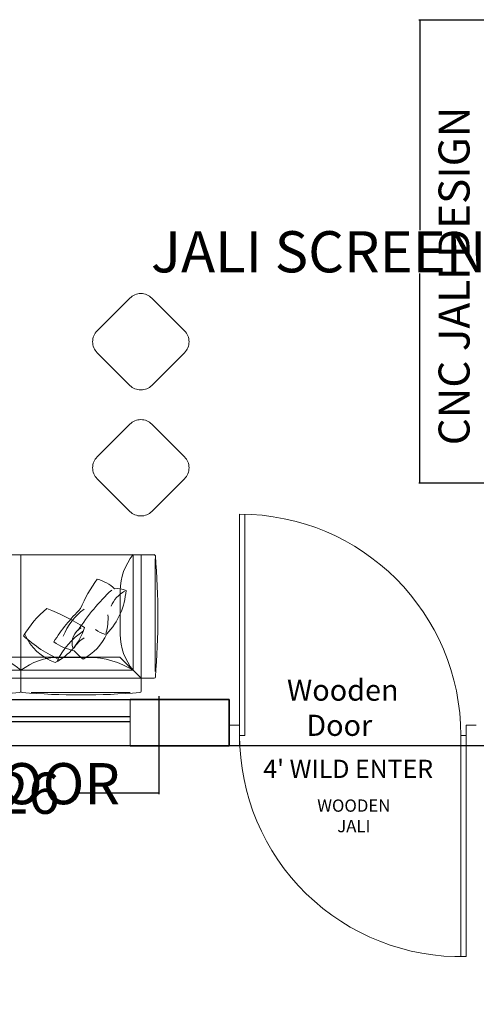
# Model space of a CAD drawing. Units: inches. Extents: x -48 to 50072, y 0 to 21068.
# Tile 50 of 75: x 123 to 212, y 628 to 819. Entities that reach past the tile are written whole.
import ezdxf

# ---------------------------------------------------------------- set-up
doc = ezdxf.new("R2010")
doc.units = ezdxf.units.IN
doc.header["$MEASUREMENT"] = 0
for name, color, linetype, lineweight in [('A-ANNO-DIMS', 2, 'Continuous', 18), ('A-ANNO-TEXT', 7, 'Continuous', 18), ('A-DOOR', 4, 'Continuous', 18), ('A-WALL', 7, 'Continuous', 35), ('FURNITURE', 44, 'Continuous', 18)]:
    doc.layers.add(name, color=color, linetype=linetype, lineweight=lineweight)
doc.layers.add('Layer3', color=176, linetype='Continuous')
doc.styles.get("Standard").update_dxf_attribs({"font": 'arial.ttf'})
doc.dimstyles.get("Standard").update_dxf_attribs({"dimtxt": 8, "dimasz": 0.18, "dimexe": 0.18, "dimexo": 0.0625, "dimgap": 0.09, "dimtad": 0, "dimtih": 1, "dimtoh": 1, "dimdec": 1, "dimzin": 0, "dimdsep": 46, "dimlunit": 4, "dimtxsty": 'Standard', "dimblk": 'ARCHTICK', "dimcen": 0.09, "dimadec": 0, "dimazin": 0, "dimtfac": 1, "dimtdec": 1, "dimtofl": 0, "dimtmove": 0, "dimatfit": 3, "dimldrblk": 'ARCHTICK', "dimfxl": 1, "dimtolj": 1, "dimtzin": 0, "dimarcsym": 0})

# ---------------------------------------------------------------- blocks, each defined once
blk = doc.blocks.new('fdsghhhhhhygr')
for p, q in [((41.77, 686.77), (41.77, 677.77)), ((144.77, 677.77), (144.77, 686.77))]:
    blk.add_line(p, q)
at = {"layer": 'Defpoints'}
for p, q in [((91.27, 683.47), (144.77, 683.47)), ((91.27, 683.47), (91.27, 682.47)), ((41.77, 682.07), (95.27, 682.07)), ((91.27, 682.47), (144.77, 682.47)), ((95.27, 682.07), (95.27, 681.07)), ((41.77, 681.07), (95.27, 681.07))]:
    blk.add_line(p, q, dxfattribs=at)
at = {"layer": 'Layer3'}
for p, q in [((41.77, 686.77), (144.77, 686.77)), ((144.77, 677.77), (41.77, 677.77))]:
    blk.add_line(p, q, dxfattribs=at)
blk = doc.blocks.new('WRG')
at = {"layer": 'FURNITURE'}
for centre, radius, start, end in [((-5881.03, 869.32), 50.97, 111.3371, 122.4176), ((-5914.7, 898.39), 23.82, 30.3068, 50.5663), ((-5895.33, 916.33), 13.61, 197.0126, 242.9429), ((-5918.49, 896.36), 18.43, 25.9005, 55.6513), ((-5915.78, 934.22), 32.17, 294.0815, 312.2768), ((-5905.57, 915.66), 12.15, 289.4501, 336.7699)]:
    blk.add_arc(centre, radius, start, end, dxfattribs=at)
blk = doc.blocks.new('DFGS')
at = {"layer": 'FURNITURE'}
for centre, radius, start, end in [((-6087.14, 813.36), 9.64, 104.9394, 132.5633), ((-6112.38, 805.26), 28.66, 21.6133, 37.4184), ((-6094.33, 816.04), 4.48, 81.3108, 116.3418), ((-6080.05, 821.2), 16.31, 184.0297, 223.6176), ((-6099.45, 813.66), 7.12, 22.214, 60.8038), ((-6126.91, 783.89), 49.66, 32.8076, 46.9), ((-6094.76, 804.41), 13.97, 20.7975, 53.8819), ((-6116.99, 784.16), 44.49, 32.4999, 45.375), ((-6080.96, 813.35), 11.17, 174.5959, 197.1556), ((-6092.61, 815.13), 5.43, 281.6061, 309.1892), ((-6087.9, 807.73), 4.17, 346.5527, 60.4145), ((-6080.21, 815.37), 12.85, 204.9913, 241.6537), ((-6089.91, 803.33), 6.58, 30.5945, 59.6065), ((-6086.56, 817.99), 12.2, 280.9279, 305.5545), ((-6095.16, 815.51), 14.47, 307.7029, 318.9387)]:
    blk.add_arc(centre, radius, start, end, dxfattribs=at)
blk = doc.blocks.new('3+2 seater sofa')
at = {"layer": 'FURNITURE'}
for p, q in [((1464.23, 900.93), (1464.23, 875.06)), ((1465.03, 901.17), (1486.94, 901.17)), ((1488.22, 900.95), (1488.22, 898.4)), ((1488.22, 898.4), (1464.22, 898.4)), ((1488.22, 898.4), (1484.13, 894.31)), ((1490.75, 898.4), (1488.22, 898.4)), ((1488.22, 898.4), (1488.22, 875.06, 0)), ((1486.69, 896.88), (1464.22, 896.88)), ((1486.69, 896.88), (1486.69, 875.06)), ((1490.98, 877.03), (1490.98, 896.27)), ((1484.13, 894.31, 0), (1464.22, 894.31)), ((1471.21, 894.37), (1479.69, 894.37)), ((1484.13, 894.31), (1484.13, 875.06)), ((1484.18, 888.22), (1484.18, 882.36)), ((1490.74, 875.06), (1464.23, 875.06)), ((1484.13, 875.06), (1490.75, 875.06)), ((1486.69, 863.06), (1486.69, 875.06)), ((1488.23, 851.03, 0), (1488.23, 875.06)), ((1490.98, 872.68), (1490.98, 863.06)), ((1484.15, 868.83), (1484.15, 863.06)), ((1484.15, 857.29), (1484.15, 863.06)), ((1484.15, 863.06, 0), (1484.15, 851.06)), ((1486.69, 863.06), (1486.69, 851.06)), ((1490.98, 853.57), (1490.98, 863.06)), ((1490.74, 851.06), (1464.23, 851.06)), ((1484.13, 851.06), (1490.75, 851.06)), ((1486.69, 839.06), (1486.69, 851.06)), ((1488.23, 827.03, 0), (1488.23, 851.06)), ((1490.98, 848.68), (1490.98, 839.06)), ((1484.15, 844.83), (1484.15, 839.06)), ((1484.15, 833.29), (1484.15, 839.06)), ((1484.15, 839.06, 0), (1484.15, 827.06)), ((1486.69, 839.06), (1486.69, 827.06)), ((1490.98, 829.57), (1490.98, 839.06)), ((1366.35, 827.06), (1392.23, 827.06)), ((1368.88, 803.07), (1368.88, 827.07)), ((1370.4, 804.59), (1370.4, 827.07)), ((1392.23, 800.54), (1392.23, 827.06)), ((1392.23, 800.54), (1392.23, 827.06)), ((1416.23, 800.54), (1416.23, 827.06)), ((1440.23, 800.54), (1440.23, 827.06)), ((1464.23, 800.54), (1464.23, 827.06)), ((1490.74, 827.06), (1464.23, 827.06)), ((1484.13, 827.06), (1490.75, 827.06)), ((1366.11, 826.25), (1366.11, 804.34)), ((1372.92, 820.07), (1372.92, 811.59)), ((1368.88, 803.07), (1372.97, 807.16)), ((1372.97, 807.16), (1392.23, 807.16)), ((1379.07, 807.11), (1384.92, 807.11)), ((1392.23, 807.16), (1392.23, 800.53)), ((1392.23, 807.16), (1392.23, 800.53)), ((1398.46, 807.13), (1404.23, 807.13)), ((1410, 807.13), (1404.23, 807.13)), ((1404.23, 807.13, 0), (1416.23, 807.13)), ((1416.23, 807.16), (1416.23, 800.53)), ((1422.46, 807.13), (1428.23, 807.13)), ((1434, 807.13), (1428.23, 807.13)), ((1428.23, 807.13, 0), (1440.23, 807.13)), ((1440.23, 807.16), (1440.23, 800.53)), ((1446.46, 807.13), (1452.23, 807.13)), ((1458, 807.13), (1452.23, 807.13)), ((1452.23, 807.13, 0), (1464.23, 807.13)), ((1464.23, 807.16), (1464.23, 800.53)), ((1370.4, 804.59), (1392.23, 804.59)), ((1404.23, 804.59), (1392.23, 804.59)), ((1404.23, 804.59), (1416.23, 804.59)), ((1428.23, 804.59), (1416.23, 804.59)), ((1428.23, 804.59), (1440.23, 804.59)), ((1452.23, 804.59), (1440.23, 804.59)), ((1452.23, 804.59), (1464.23, 804.59)), ((1366.33, 803.07), (1368.88, 803.07)), ((1368.88, 800.53), (1368.88, 803.07)), ((1368.88, 803.07), (1392.23, 803.07, 0)), ((1416.26, 803.06, 0), (1392.23, 803.06)), ((1440.26, 803.06, 0), (1416.23, 803.06)), ((1464.26, 803.06, 0), (1440.23, 803.06)), ((1390.25, 800.3), (1371.02, 800.3)), ((1394.6, 800.3), (1404.23, 800.3)), ((1413.72, 800.3), (1404.23, 800.3)), ((1418.6, 800.3), (1428.23, 800.3)), ((1437.72, 800.3), (1428.23, 800.3)), ((1442.6, 800.3), (1452.23, 800.3)), ((1461.72, 800.3), (1452.23, 800.3))]:
    blk.add_line(p, q, dxfattribs=at)
at = {"layer": 'FURNITURE', "ltscale": 3}
for p, q in [((1464.23, 875.06), (1464.23, 851.06)), ((1484.15, 863.06), (1484.15, 875.06)), ((1484.15, 863.06), (1484.15, 851.06)), ((1464.23, 851.06), (1464.23, 827.06)), ((1484.15, 839.06), (1484.15, 851.06)), ((1484.15, 839.06), (1484.15, 827.06)), ((1392.23, 827.06), (1416.23, 827.06)), ((1416.23, 827.06), (1440.23, 827.06)), ((1440.23, 827.06), (1464.23, 827.06)), ((1404.23, 807.13), (1392.23, 807.13)), ((1404.23, 807.13), (1416.23, 807.13)), ((1428.23, 807.13), (1416.23, 807.13)), ((1428.23, 807.13), (1440.23, 807.13)), ((1452.23, 807.13), (1440.23, 807.13)), ((1452.23, 807.13), (1464.23, 807.13))]:
    blk.add_line(p, q, dxfattribs=at)
at = {"layer": 'FURNITURE'}
for centre, radius, start, end in [((1476.31, 758.13), 143.55, 85.3368, 94.7395), ((1464.47, 900.93), 0.255, 94.7915, 180), ((1487.96, 900.95), 0.255, 0, 85.2857), ((1490.75, 898.15), 0.255, 5.7807, 90), ((1354.3, 886.73), 137.18, 355.2142, 4.7858), ((1471.31, 905.62), 11.26, 230.9515, 269.5157), ((1479.6, 905.62), 11.26, 270.4843, 309.0485), ((1500.6, 888.15), 16.42, 147.8787, 179.7559), ((1496.3, 882.45), 12.13, 180.424, 217.563), ((1493.43, 868.68), 9.28, 136.5598, 179.0844), ((1490.74, 874.8), 0.255, 4.5067, 90), ((1490.75, 875.31), 0.255, 270, 354.2193), ((1348.3, 862.96), 143.19, 0.0378, 4.7508), ((1348.3, 863.15), 143.19, 355.2492, 359.9622), ((1493.43, 857.43), 9.28, 180.9156, 223.4402), ((1493.43, 844.68), 9.28, 136.5598, 179.0844), ((1490.74, 851.31), 0.255, 270, 355.4933), ((1348.3, 838.96), 143.19, 0.0378, 4.7508), ((1348.3, 839.15), 143.19, 355.2492, 359.9622), ((1493.43, 833.43), 9.28, 180.9156, 223.4402), ((1509.16, 814.97), 143.55, 175.2605, 184.6632), ((1366.35, 826.81), 0.255, 90, 175.2085), ((1361.66, 819.98), 11.26, 0.4843, 39.0485), ((1490.74, 827.31), 0.255, 270, 355.4933), ((1361.66, 811.68), 11.26, 320.9515, 359.5157), ((1379.14, 790.68), 16.42, 90.2441, 122.1213), ((1384.83, 794.98), 12.13, 52.437, 89.576), ((1398.61, 797.86), 9.28, 90.9156, 133.4402), ((1409.85, 797.86), 9.28, 46.5598, 89.0844), ((1422.61, 797.86), 9.28, 90.9156, 133.4402), ((1433.85, 797.86), 9.28, 46.5598, 89.0844), ((1446.61, 797.86), 9.28, 90.9156, 133.4402), ((1457.85, 797.86), 9.28, 46.5598, 89.0844), ((1366.33, 803.32), 0.255, 184.7143, 270), ((1369.13, 800.53), 0.255, 180, 264.2193), ((1380.55, 936.98), 137.18, 265.2142, 274.7858), ((1391.97, 800.54), 0.255, 274.5067, 0), ((1391.97, 800.53), 0.255, 275.7807, 0), ((1392.48, 800.54), 0.255, 180, 265.4933), ((1392.48, 800.53), 0.255, 180, 264.2193), ((1404.32, 942.98), 143.19, 265.2492, 269.9622), ((1404.13, 942.98), 143.19, 270.0378, 274.7508), ((1415.97, 800.54), 0.255, 274.5067, 0), ((1428.32, 942.98), 143.19, 265.2492, 269.9622), ((1428.13, 942.98), 143.19, 270.0378, 274.7508), ((1439.97, 800.54), 0.255, 274.5067, 0), ((1452.32, 942.98), 143.19, 265.2492, 269.9622), ((1452.13, 942.98), 143.19, 270.0378, 274.7508), ((1463.97, 800.54), 0.255, 274.5067, 0)]:
    blk.add_arc(centre, radius, start, end, dxfattribs=at)
at = {"layer": 'FURNITURE', "yscale": 0.8336162403020807, "zscale": 0.8336162403020807}
for name, p, xscale, rotation in [('DFGS', (2154.78, -4186.5, 0), -0.8336162403020807, 90), ('WRG', (2238.95, -4037.88), -0.8336162403020807, 90), ('DFGS', (-2239.7, -2654.91), -0.8336162403020807, 35.78436137719967), ('DFGS', (-2239.7, -2678.91), -0.8336162403020807, 35.78436137719967), ('DFGS', (4922.38, 4530.98), 0.8336162403020807, 54.21563862280032), ('DFGS', (4946.38, 4530.98), 0.8336162403020807, 54.21563862280032), ('DFGS', (4970.38, 4530.98), 0.8336162403020807, 54.21563862280032)]:
    blk.add_blockref(name, p, dxfattribs=dict(at, xscale=xscale, rotation=rotation))
at = {"layer": 'FURNITURE', "xscale": 0.8336162403020807, "yscale": 0.8336162403020807, "zscale": 0.8336162403020807}
for name, p in [('DFGS', (6453.79, 136.5, 0)), ('WRG', (6305.16, 52.33))]:
    blk.add_blockref(name, p, dxfattribs=at)
blk = doc.blocks.new('DOOR-ENTRY-TANDEM-48')
for p, q in [((2, 43), (2, 86)), ((3, 85.99), (3, 43)), ((0, 45), (2, 45)), ((2, 41), (2, 45)), ((46, 41), (46, 45)), ((46, 45), (48, 45)), ((2, 43), (3, 43)), ((2, 43), (3, 43)), ((2, 43), (3, 43)), ((45, 0), (45, 43)), ((45, 43), (46, 43)), ((46, 43), (46, 7)), ((0, 41), (48, 41)), ((46, 7), (46, 0.01))]:
    blk.add_line(p, q)
for centre, start, end in [((2, 43), 0, 90), ((45, 43), 180, 271.3326)]:
    blk.add_arc(centre, 43, start, end)
blk = doc.blocks.new('_ArchTick')
at = {"color": 0, "linetype": 'ByBlock', "const_width": 0.15}
blk.add_lwpolyline([(-0.5, -0.5), (0.5, 0.5)], dxfattribs=at)
blk = doc.blocks.new('*D68')
at = {"layer": 'A-ANNO-DIMS', "color": 0, "lineweight": -2, "transparency": 16777216}
for p, q in [((257.08, 632.91), (262.77, 632.91)), ((262.59, 632.91), (262.59, 618.57)), ((262.59, 595.77), (262.59, 610.11)), ((257.08, 595.77), (262.77, 595.77))]:
    blk.add_line(p, q, dxfattribs=at)
at = {"layer": 'Defpoints', "color": 0, "transparency": 16777216}
for p in [(257.02, 632.91), (257.02, 595.77), (262.59, 595.77)]:
    blk.add_point(p, dxfattribs=at)
at = {"layer": 'A-ANNO-DIMS', "color": 0, "lineweight": -2, "transparency": 16777216, "xscale": 0.18, "yscale": 0.18, "zscale": 0.18}
for p, rotation in [((262.59, 632.91), 90), ((262.59, 595.77), 270)]:
    blk.add_blockref('_ArchTick', p, dxfattribs=dict(at, rotation=rotation))
at = {"layer": 'A-ANNO-DIMS', "color": 0, "transparency": 16777216, "insert": (262.59, 614.34), "char_height": 8, "attachment_point": 5}
blk.add_mtext('\\A1;TOILET DOOR A 37 TYP.', dxfattribs=at)
blk = doc.blocks.new('*D100')
at = {"layer": 'A-ANNO-DIMS', "color": 0, "lineweight": -2, "transparency": 16777216}
for p, q in [((214.45, 818.77), (200.84, 818.77)), ((201.02, 818.77), (201.02, 778)), ((201.02, 728.77), (201.02, 769.55)), ((214.45, 728.77), (200.84, 728.77))]:
    blk.add_line(p, q, dxfattribs=at)
at = {"layer": 'Defpoints', "color": 0, "transparency": 16777216}
for p in [(201.02, 818.77), (214.52, 818.77), (214.52, 728.77)]:
    blk.add_point(p, dxfattribs=at)
at = {"layer": 'A-ANNO-DIMS', "color": 0, "lineweight": -2, "transparency": 16777216, "xscale": 0.18, "yscale": 0.18, "zscale": 0.18}
for p, rotation in [((201.02, 818.77), 90), ((201.02, 728.77), 270)]:
    blk.add_blockref('_ArchTick', p, dxfattribs=dict(at, rotation=rotation))
at = {"layer": 'A-ANNO-DIMS', "color": 0, "transparency": 16777216, "insert": (201.02, 773.77), "char_height": 8, "attachment_point": 5}
blk.add_mtext('\\A1;JALI SCREEN 90 TYP.', dxfattribs=at)
blk = doc.blocks.new('*D108')
at = {"layer": 'A-ANNO-DIMS', "color": 0, "lineweight": -2, "transparency": 16777216}
for p, q in [((24.1, 687.42), (24.1, 668.37)), ((150.3, 687.42), (150.3, 668.37)), ((24.1, 668.55), (39.48, 668.55)), ((150.3, 668.55), (134.91, 668.55))]:
    blk.add_line(p, q, dxfattribs=at)
at = {"layer": 'Defpoints', "color": 0, "transparency": 16777216}
for p in [(24.1, 687.48), (150.3, 687.48), (24.1, 668.55)]:
    blk.add_point(p, dxfattribs=at)
at = {"layer": 'A-ANNO-DIMS', "color": 0, "lineweight": -2, "transparency": 16777216, "xscale": 0.18, "yscale": 0.18, "zscale": 0.18, "rotation": 180}
blk.add_blockref('_ArchTick', (24.1, 668.55), dxfattribs=at)
at = {"layer": 'A-ANNO-DIMS', "color": 0, "lineweight": -2, "transparency": 16777216, "xscale": 0.18, "yscale": 0.18, "zscale": 0.18}
blk.add_blockref('_ArchTick', (150.3, 668.55), dxfattribs=at)
at = {"layer": 'A-ANNO-DIMS', "color": 0, "transparency": 16777216, "insert": (87.2, 668.55), "char_height": 8, "attachment_point": 5}
blk.add_mtext('\\A1;SOFA GROUP 126', dxfattribs=at)
blk = doc.blocks.new('*D116')
at = {"layer": 'A-ANNO-DIMS', "color": 0, "lineweight": -2, "transparency": 16777216}
for p, q in [((18.02, 677.71), (18.02, 165.94)), ((216.02, 677.71), (216.02, 165.94)), ((18.02, 166.12), (108.46, 166.12)), ((216.02, 166.12), (125.58, 166.12))]:
    blk.add_line(p, q, dxfattribs=at)
at = {"layer": 'Defpoints', "color": 0, "transparency": 16777216}
for p in [(18.02, 677.77), (216.02, 677.77), (216.02, 166.12)]:
    blk.add_point(p, dxfattribs=at)
at = {"layer": 'A-ANNO-DIMS', "color": 0, "lineweight": -2, "transparency": 16777216, "xscale": 0.18, "yscale": 0.18, "zscale": 0.18, "rotation": 180}
blk.add_blockref('_ArchTick', (18.02, 166.12), dxfattribs=at)
at = {"layer": 'A-ANNO-DIMS', "color": 0, "lineweight": -2, "transparency": 16777216, "xscale": 0.18, "yscale": 0.18, "zscale": 0.18}
blk.add_blockref('_ArchTick', (216.02, 166.12), dxfattribs=at)
at = {"layer": 'A-ANNO-DIMS', "color": 0, "transparency": 16777216, "insert": (117.02, 166.12), "char_height": 8, "attachment_point": 5}
blk.add_mtext('\\A1;198', dxfattribs=at)
blk = doc.blocks.new('*D127')
at = {"layer": 'A-ANNO-DIMS', "color": 0, "lineweight": -2, "transparency": 16777216}
for p, q in [((215.95, 677.77), (-34.61, 677.77)), ((-34.43, 677.77), (-34.43, 587.45)), ((-34.43, 488.77), (-34.43, 579.1)), ((215.95, 488.77), (-34.61, 488.77))]:
    blk.add_line(p, q, dxfattribs=at)
at = {"layer": 'Defpoints', "color": 0, "transparency": 16777216}
for p in [(-34.43, 677.77), (216.02, 677.77), (216.02, 488.77)]:
    blk.add_point(p, dxfattribs=at)
at = {"layer": 'A-ANNO-DIMS', "color": 0, "lineweight": -2, "transparency": 16777216, "xscale": 0.18, "yscale": 0.18, "zscale": 0.18}
for p, rotation in [((-34.43, 677.77), 90), ((-34.43, 488.77), 270)]:
    blk.add_blockref('_ArchTick', p, dxfattribs=dict(at, rotation=rotation))
at = {"layer": 'A-ANNO-DIMS', "color": 0, "transparency": 16777216, "insert": (-34.43, 583.27), "char_height": 8, "attachment_point": 5}
blk.add_mtext('\\A1;189', dxfattribs=at)

msp = doc.modelspace()

# ---------------------------------------------------------------- linework, layer by layer
at = {"layer": 'A-WALL'}
for p, q in [((164.017, 686.775), (144.768, 686.775)), ((164.017, 677.775), (164.017, 686.775)), ((164.017, 677.775), (144.768, 677.775))]:
    msp.add_line(p, q, dxfattribs=at)
at = {"layer": 'FURNITURE'}
for points in [[(155.306, 754.161), (148.942, 747.797, -0.4142136), (144.699, 747.797), (138.335, 754.161, -0.4142136), (138.335, 758.404), (144.699, 764.768, -0.4142136), (148.942, 764.768), (155.306, 758.404, -0.4142136)], [(155.306, 733.912), (148.942, 740.275, 0.4142136), (144.699, 740.275), (138.335, 733.912, 0.4142136), (138.335, 729.669), (144.699, 723.305, 0.4142136), (148.942, 723.305), (155.306, 729.669, 0.4142136)]]:
    msp.add_lwpolyline(points, format="xyb", close=True, dxfattribs=at)

# ---------------------------------------------------------------- block references
at = {"layer": 'A-DOOR'}
for name, p in [('DOOR-ENTRY-TANDEM-48', (164.017, 636.775)), ('fdsghhhhhhygr', (0, 0))]:
    msp.add_blockref(name, p, dxfattribs=at)
at = {"layer": 'FURNITURE', "xscale": -1}
msp.add_blockref('3+2 seater sofa', (1515.738, -112.158), dxfattribs=at)

# ---------------------------------------------------------------- texts
at = {"layer": 'A-ANNO-TEXT', "insert": (204.677, 736.172), "char_height": 6.02726, "attachment_point": 1, "rotation": 90}
msp.add_mtext_dynamic_manual_height_columns('CNC JALI DESIGN ', width=285.38642, gutter_width=30.136, heights=[0], dxfattribs=at)
at = {"layer": 'A-ANNO-TEXT', "attachment_point": 1}
for s, width, gutter_width, insert, char_height in [('Wooden^J   Door', 42.42894, 20.514, (175.22, 690.633), 4.10286), ('UPVC SLIDING DOOR ', 126.59735, 40, (37.479, 674.399), 8), ("4' WILD ENTER", 45.36164, 17.739, (170.616, 675.05), 3.5477), ('\\pxqc;WOODEN^JJALI', 27.24055, 11.943, (174.592, 667.332), 2.38857)]:
    msp.add_mtext_dynamic_manual_height_columns(s, width=width, gutter_width=gutter_width, heights=[0], dxfattribs=dict(at, insert=insert, char_height=char_height))

# ---------------------------------------------------------------- dimensions: what is measured, and where the dimension line sits
at = {"layer": 'A-ANNO-DIMS'}
for base, p1, p2, angle, text, picture, middle in [((201.017, 818.775), (214.517, 728.775), (214.517, 818.775), 90, 'JALI SCREEN <> TYP.', '*D100', (201.017, 773.775)), ((24.097, 668.554), (150.298, 687.484), (24.097, 687.484), 180, 'SOFA GROUP <>', '*D108', (87.197, 668.554)), ((262.588, 595.775), (257.017, 632.911), (257.017, 595.775), 270, 'TOILET DOOR A <> TYP.', '*D68', (262.588, 614.343))]:
    dim = msp.add_linear_dim(base=base, p1=p1, p2=p2, angle=angle, text=text, dimstyle='Standard', override={"dimdec": 0, "dimlfac": 1, "dimrnd": 0, "dimzin": 0, "dimdsep": 46, "dimlunit": 2}, dxfattribs=at)
    dim.commit()
    dim.dimension.update_dxf_attribs({"geometry": picture, "text_midpoint": middle})
dim = msp.add_linear_dim(base=(-34.433, 677.775), p1=(216.017, 488.775), p2=(216.017, 677.775), angle=90, dimstyle='Standard', override={"dimdec": 0, "dimlfac": 1, "dimrnd": 0, "dimzin": 0, "dimdsep": 46, "dimlunit": 2}, dxfattribs=at)
dim.commit()
dim.dimension.update_dxf_attribs({"geometry": '*D127', "text_midpoint": (-34.433, 583.275)})
dim = msp.add_linear_dim(base=(216.017, 166.125), p1=(18.017, 677.775), p2=(216.017, 677.775), dimstyle='Standard', override={"dimdec": 0, "dimlfac": 1, "dimrnd": 0, "dimzin": 0, "dimdsep": 46, "dimlunit": 2}, dxfattribs=at)
dim.commit()
dim.dimension.update_dxf_attribs({"geometry": '*D116', "text_midpoint": (117.017, 166.125)})

doc.saveas('drawing.dxf')
